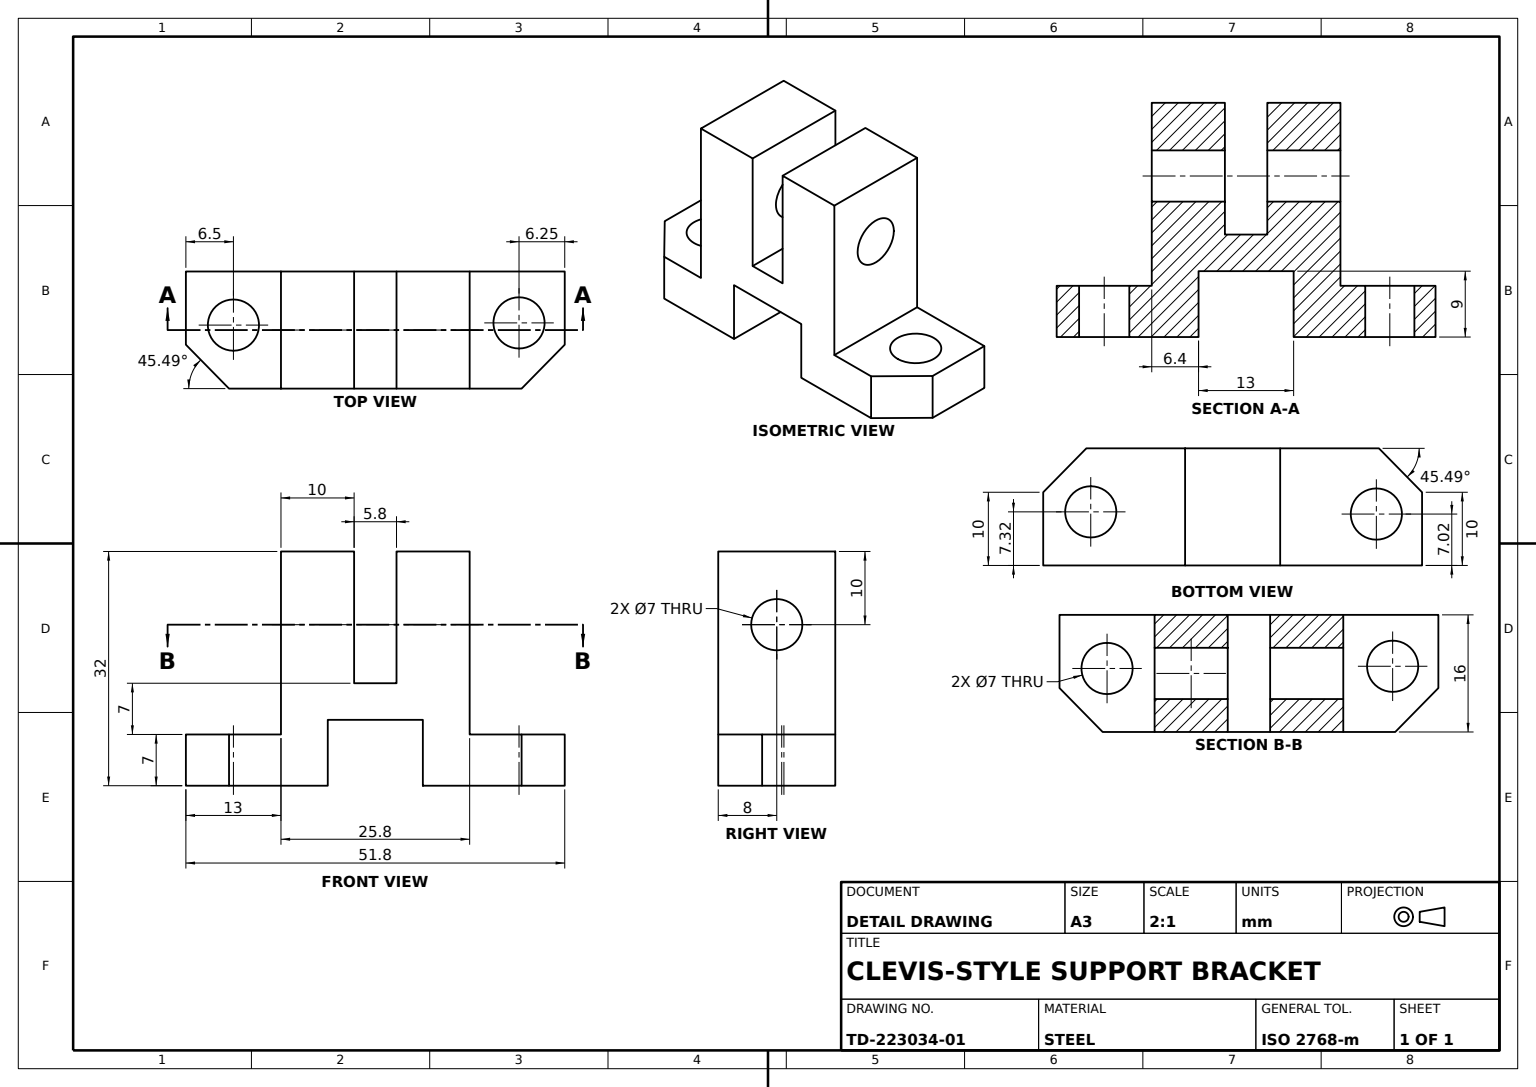
SolidWorks part; units mm, degrees
material "Plain Carbon Steel"
ref_plane "Front Plane" through (0, 0, 0) normal (0, 0, 1) x (1, 0, 0)
ref_plane "Top Plane" through (0, 0, 0) normal (0, 1, 0) x (1, 0, 0)
ref_plane "Right Plane" through (0, 0, 0) normal (1, 0, 0) x (0, 0, -1)
sketch "Base Plate Sketch" plane through (0, 0, 0) normal (0, 1, 0) x (1, 0, 0)
  line L0 (-51.797, -2.1971) -> (-51.797, -12.1971)
  line L2 (-45.8985, -18.1971) -> (-5.8985, -18.1971)
  line L4 (0, -12.1971) -> (0, -2.1971)
  line L5 (-51.797, -2.1971) -> (0, -2.1971)
  line L6 (-45.8985, -18.1971) -> (-51.797, -12.1971)
  line L7 (-5.8985, -18.1971) -> (0, -12.1971)
  point P2 (-25.8985, -18.1971)
  point P8 (-25.8985, -2.1971)
  dimension "D1" = 10
  dimension "D2" = 10
  dimension "D3" = 40
  dimension "D4" = 0
  dimension "D5" = 16
  dimension "D6" = 51.797
  dimension "D7" = 2.1971
extrude "Base Plate" add sketch "Base Plate Sketch" along normal blind 7
sketch "Base Relief Cut Sketch" plane through (0, 7, 0) normal (0, 1, 0) x (1, 0, 0)
  line L0 (-51.797, -2.1971) -> (-38.797, -2.1971)
  line L1 (0, -2.1971) -> (-51.797, -2.1971) construction
  circle A0 centre (-45.297, -9.5197) radius 3.5
  point P9 (-45.297, -2.1971)
  dimension "D1" = 7
  dimension "D2" = 13
  dimension "D3" = 0
  dimension "D4" = 7.3226
extrude "Base Relief Cut" cut sketch "Base Relief Cut Sketch" against normal blind 18 and the other way blind 16 contours A0
sketch "Base Trim Cut Sketch" plane through (0, 7, 0) normal (0, 1, 0) x (1, 0, 0)
  line L0 (0, -2.1971) -> (-12.501, -2.1971)
  line L1 (0, -2.1971) -> (-51.797, -2.1971) construction
  line L2 (-51.797, -2.1971) -> (-51.797, -12.1971) construction
  circle A0 centre (-6.2505, -9.2186) radius 3.5
  point P8 (-6.2505, -2.1971)
  dimension "D1" = 7
  dimension "D2" = 39.2959
  dimension "D3" = 7.0215
extrude "Base Trim Cut" cut sketch "Base Trim Cut Sketch" against normal blind 35 and the other way blind 27 contours A0
sketch "Upright Block Sketch 13x13" plane through (0, 7, 0) normal (0, 1, 0) x (1, 0, 0)
  line L0 (-38.797, -18.1971) -> (-38.797, -2.1971)
  line L1 (-45.8985, -18.1971) -> (-5.8985, -18.1971) construction
  line L2 (0, -2.1971) -> (-51.797, -2.1971) construction
  line L3 (-38.797, -2.1971) -> (-13, -2.1971)
  line L4 (-13, -2.1971) -> (-13, -18.1971)
  line L5 (-13, -18.1971) -> (-38.797, -18.1971)
  dimension "D1" = 13
  dimension "D2" = 13
extrude "Upright Block" add sketch "Upright Block Sketch 13x13" along normal blind 25
sketch "Upright Slot Sketch" plane through (0, 0, 18.1971) normal (0, 0, 1) x (1, 0, 0)
  line L0 (-28.797, 32) -> (-28.797, 22.2471)
  line L1 (-38.797, 32) -> (-13, 32) construction
  line L2 (-23, 32) -> (-23, 14)
  line L3 (-28.797, 22.2471) -> (-28.797, 14)
  line L4 (-23, 14) -> (-28.797, 14)
  line L5 (-28.797, 32) -> (-23, 32)
  line L7 (-45.8985, 0) -> (-5.8985, 0) construction
  dimension "D1" = 10
  dimension "D2" = 10
  dimension "D3" = 14
  dimension "D4" = 22.2471
extrude "Upright Slot" cut sketch "Upright Slot Sketch" against normal blind 84 and the other way blind 38
sketch "Upright Cross Hole Sketch" plane through (-13, 0, 0) normal (1, 0, 0) x (0, 0, -1)
  line L1 (-2.1971, 32) -> (-2.1971, 7) construction
  circle A0 centre (-10.1971, 22) radius 3.5
  dimension "D1" = 7
  dimension "D2" = 10
  dimension "D3" = 8
extrude "Upright Cross Hole" cut sketch "Upright Cross Hole Sketch" along normal blind 10 and the other way blind 13
sketch "Through Hole Sketch" plane through (-28.797, 0, 0) normal (1, 0, 0) x (0, 0, -1)
  circle A0 centre (-10.1971, 22) radius 3.5
  dimension "D1" = 7
extrude "Through Hole" cut sketch "Through Hole Sketch" against normal blind 14
sketch "Base Clearance Cut Sketch" plane through (0, 0, 18.1971) normal (0, 0, 1) x (1, 0, 0)
  line L0 (-32.3985, 0) -> (-32.3985, 9)
  line L1 (-45.8985, 0) -> (-5.8985, 0) construction
  line L2 (-19.3985, 0) -> (-19.3985, 9)
  line L3 (-28.797, 14) -> (-23, 14) construction
  line L4 (-32.3985, 9) -> (-19.3985, 9)
  line L5 (-32.3985, 0) -> (-19.3985, 0)
  point P8 (-25.8985, 14)
  dimension "D1" = 9
  dimension "D2" = 9
  dimension "D3" = 6.5
  dimension "D4" = 6.5
extrude "Base Clearance Cut" cut sketch "Base Clearance Cut Sketch" against normal blind 58 and the other way blind 17
